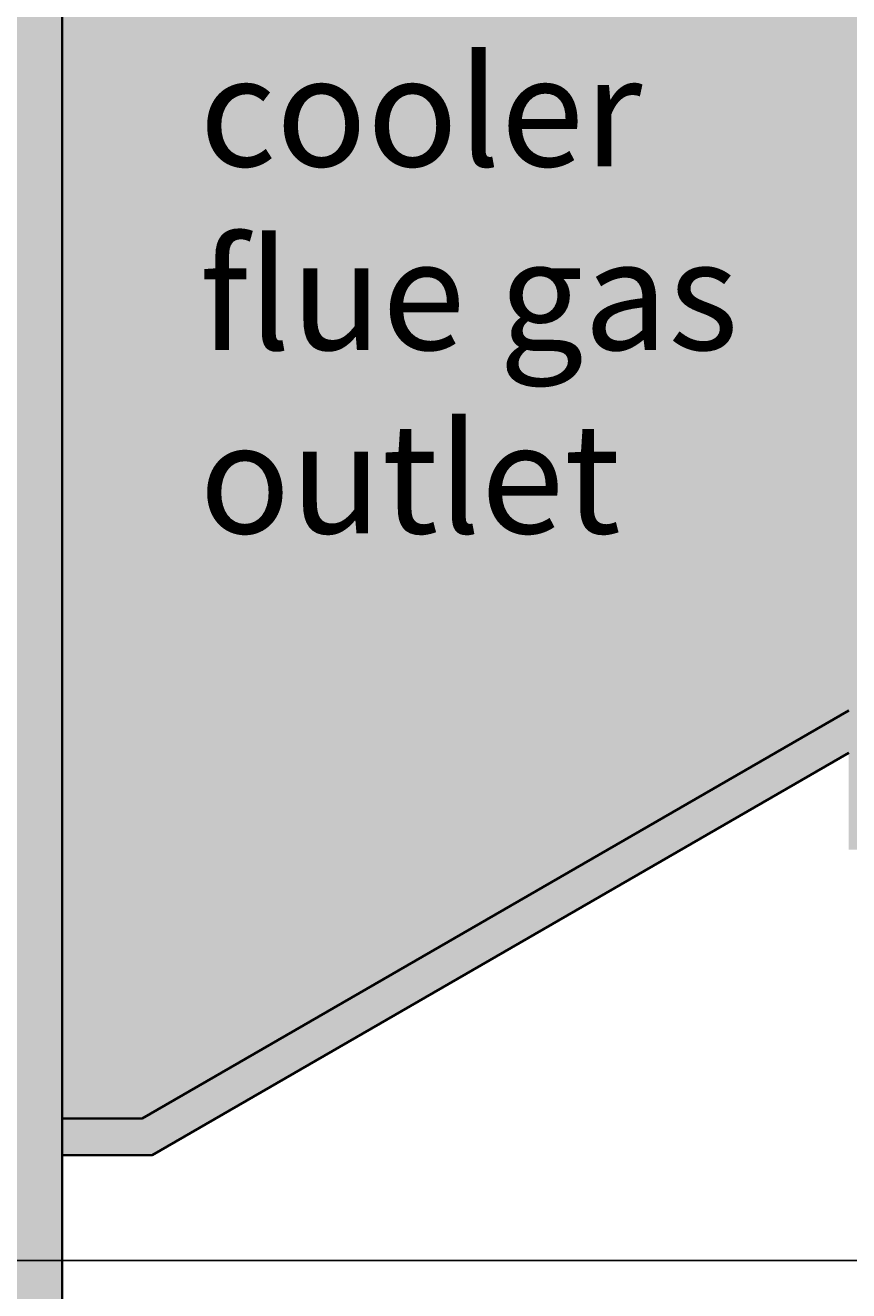
# Model space of a CAD drawing. Units: inches. Extents: x -1 to 292, y -3 to 199.
# Tile 38 of 52: x 181 to 203, y 43 to 77. Entities that reach past the tile are written whole.
import ezdxf

# ---------------------------------------------------------------- set-up
doc = ezdxf.new("R2010")
doc.units = ezdxf.units.IN
doc.header["$MEASUREMENT"] = 0
for name, color, linetype, lineweight in [('M-ANNO-TEXT', 3, 'Continuous', 25), ('M-DIMS', 2, 'Continuous', 18), ('M-EQPM', 7, 'Continuous', 35), ('M-PATT', 8, 'Continuous', 13)]:
    doc.layers.add(name, color=color, linetype=linetype, lineweight=lineweight)
doc.styles.get("Standard").update_dxf_attribs({"font": 'arial.ttf'})
doc.dimstyles.get("Standard").update_dxf_attribs({"dimtxt": 0.18, "dimasz": 0.18, "dimexe": 0.18, "dimexo": 0.0625, "dimgap": 0.09, "dimtad": 0, "dimtih": 1, "dimtoh": 1, "dimdec": 4, "dimzin": 0, "dimdsep": 46, "dimtxsty": 'Standard', "dimcen": 0.09, "dimadec": 0, "dimazin": 0, "dimtfac": 1, "dimtdec": 4, "dimtofl": 0, "dimtmove": 0, "dimatfit": 3, "dimfxl": 1, "dimtolj": 1, "dimtzin": 0, "dimarcsym": 0})

# ---------------------------------------------------------------- blocks, each defined once
blk = doc.blocks.new('*D7')
at = {"layer": 'Defpoints', "color": 0, "transparency": 16777216}
for p in [(21.861, 54.582), (205.115, 54.582), (21.861, 39.982)]:
    blk.add_point(p, dxfattribs=at)
at = {"layer": 'M-DIMS', "color": 0, "lineweight": -2, "transparency": 16777216}
for p, q in [((21.861, 54.52), (21.861, 39.802)), ((205.115, 54.52), (205.115, 39.802)), ((22.041, 39.982), (113.033, 39.982)), ((204.935, 39.982), (113.944, 39.982))]:
    blk.add_line(p, q, dxfattribs=at)
at = {"layer": 'M-DIMS', "color": 0, "transparency": 16777216}
for points in [[(22.041, 40.012), (22.041, 39.952), (21.861, 39.982)], [(204.935, 40.012), (204.935, 39.952), (205.115, 39.982)]]:
    blk.add_solid(points, dxfattribs=at)
at = {"layer": 'M-DIMS', "color": 0, "transparency": 16777216, "insert": (113.488, 39.982), "char_height": 0.18, "attachment_point": 5}
blk.add_mtext('\\A1;183.25', dxfattribs=at)
blk = doc.blocks.new('*D10')
at = {"layer": 'Defpoints', "color": 0, "transparency": 16777216}
for p in [(169.176, 99.774), (169.176, 43.391), (292.04, 43.391)]:
    blk.add_point(p, dxfattribs=at)
at = {"layer": 'M-DIMS', "color": 0, "lineweight": -2, "transparency": 16777216}
for p, q in [((169.239, 99.774), (292.22, 99.774)), ((292.04, 99.594), (292.04, 71.764)), ((292.04, 43.571), (292.04, 71.4)), ((169.239, 43.391), (292.22, 43.391))]:
    blk.add_line(p, q, dxfattribs=at)
at = {"layer": 'M-DIMS', "color": 0, "transparency": 16777216}
for points in [[(292.01, 99.594), (292.07, 99.594), (292.04, 99.774)], [(292.01, 43.571), (292.07, 43.571), (292.04, 43.391)]]:
    blk.add_solid(points, dxfattribs=at)
at = {"layer": 'M-DIMS', "color": 0, "transparency": 16777216, "insert": (292.04, 71.582), "char_height": 0.18, "attachment_point": 5}
blk.add_mtext('\\A1;56.38', dxfattribs=at)

msp = doc.modelspace()

# ---------------------------------------------------------------- hatches: boundary and pattern name
at = {"layer": 'M-PATT'}
h = msp.add_hatch(color=256, dxfattribs=at)
h.set_gradient(color1=(0, 127, 0), color2=(0, 127, 0), tint=1, name='CYLINDER')
h.paths.add_polyline_path([(164.5186, 119.2985), (129.9293, 119.2985), (129.9293, 117.2985), (164.1897, 117.2985)])
h.paths.add_polyline_path([(181.5897, 119.2985), (164.5186, 119.2985), (164.1897, 117.2985), (179.5897, 117.2985), (179.5897, 107.8518), (181.5897, 109.1506)])
h.paths.add_polyline_path([(181.5897, 109.1506), (179.5897, 107.8518), (179.5897, 36.2698), (198.4159, 36.2698), (198.4159, 38.2698), (181.5897, 38.2698)])
h.paths.add_polyline_path([(115.4883, 126.765), (111.4883, 126.765), (111.4883, 114.6589), (115.4883, 114.6589)])
h.paths.add_polyline_path([(123.408, 119.2985), (115.4883, 119.2985), (115.4883, 117.2985), (123.408, 117.2985)])
h.paths.add_polyline_path([(115.4883, 112.6589), (111.4883, 112.6589), (111.4883, 106.9941), (115.4883, 106.9941)])
h.paths.add_polyline_path([(120.9032, 106.9941), (106.0735, 106.9941), (106.0735, 105.9941), (120.9032, 105.9941)])
h.paths.add_polyline_path([(236.4209, 117.5104), (234.9209, 117.5104), (234.9209, 97.1861), (236.4209, 97.1861)])
h.paths.add_polyline_path([(236.4209, 126.4904), (234.9209, 126.4904), (234.9209, 118.9331), (236.4209, 118.9331)])
h.paths.add_polyline_path([(244.9552, 125.7269), (242.9552, 125.7269), (242.9552, 116.8562), (244.9552, 116.8562)])
h.paths.add_polyline_path([(244.9552, 115.1721), (242.9552, 115.1721), (242.9552, 109.7385), (244.9552, 109.7385)])
h.paths.add_polyline_path([(248.4468, 109.7385), (239.4637, 109.7385), (239.4637, 109.4289), (248.4468, 109.4289)])
h = msp.add_hatch(color=256, dxfattribs=at)
h.set_gradient(color1=(237, 31, 36), color2=(242, 113, 114), tint=1, name='CYLINDER')
h.paths.add_polyline_path([(106.0735, 105.9941), (106.0735, 106.9941), (108.0603, 106.9941), (107.8488, 107.6501), (57.8007, 107.6501, 0.4142136), (49.9241, 99.7735), (52.3176, 101.3278), (55.0097, 99.7735), (57.4032, 101.3278), (60.0953, 99.7735), (62.4888, 101.3278), (65.1809, 99.7735), (67.5744, 101.3278), (70.2665, 99.7735), (72.66, 101.3278), (75.3521, 99.7735), (77.7456, 101.3278), (80.4377, 99.7735), (82.8312, 101.3278), (85.5233, 99.7735), (87.9168, 101.3278), (90.6089, 99.7735), (93.0024, 101.3278), (95.6945, 99.7735), (98.088, 101.3278), (100.7801, 99.7735), (103.1736, 101.3278), (105.8657, 99.7735), (108.2592, 101.3278), (110.9513, 99.7735), (113.3448, 101.3278), (116.0369, 99.7735), (118.4304, 101.3278), (121.1225, 99.7735), (123.516, 101.3278), (126.2082, 99.7735), (128.6016, 101.3278), (131.2938, 99.7735), (133.6872, 101.3278), (136.3794, 99.7735), (138.7728, 101.3278), (141.465, 99.7735), (143.8584, 101.3278), (146.5506, 99.7735), (148.944, 101.3278), (151.6362, 99.7735), (154.0296, 101.3278), (156.7218, 99.7735), (159.1152, 101.3278), (160.6222, 100.4578), (160.6222, 107.6501), (115.4883, 107.6501), (115.4883, 106.9941), (120.9032, 106.9941), (120.9032, 105.9941), (120.9032, 103.3981), (106.0735, 103.3981)])
h.paths.add_polyline_path([(169.176, 107.6501), (162.1623, 107.6501), (162.1623, 100.004), (164.2008, 101.3278), (166.893, 99.7735), (169.2864, 101.3278), (171.9786, 99.7735), (174.372, 101.3278), (177.0526, 99.7802, 0.4139642)])
h.paths.add_polyline_path([(111.4883, 107.6501), (107.8488, 107.6501), (108.0603, 106.9941), (111.4883, 106.9941)], flags=17)
h.paths.add_polyline_path([(61.6788, 91.897), (57.8007, 91.897, -0.1099266), (54.4604, 92.6403), (43.2011, 92.6403), (23.9502, 84.4688), (23.9502, 58.376), (43.2011, 47.2615), (50.9409, 47.2615, -0.2705926), (57.8007, 51.2672), (61.6788, 51.2672)])
h.paths.add_polyline_path([(73.6788, 91.897), (70.6788, 91.897), (70.6788, 51.2672), (73.6788, 51.2672)])
h.paths.add_polyline_path([(79.6788, 91.897), (76.6788, 91.897), (76.6788, 51.2672), (79.6788, 51.2672)])
h.paths.add_polyline_path([(67.6788, 91.897), (64.6788, 91.897), (64.6788, 51.2672), (67.6788, 51.2672)])
h.paths.add_polyline_path([(101.6788, 91.897), (82.6788, 91.897), (82.6788, 51.2672), (101.6788, 51.2672)])
h.paths.add_polyline_path([(107.6788, 91.897), (104.6788, 91.897), (104.6788, 51.2672), (107.6788, 51.2672)])
h.paths.add_polyline_path([(113.6788, 91.897), (110.6788, 91.897), (110.6788, 51.2672), (113.6788, 51.2672)])
h.paths.add_polyline_path([(119.6788, 91.897), (116.6788, 91.897), (116.6788, 51.2672), (119.6788, 51.2672)])
h.paths.add_polyline_path([(141.6788, 91.897), (122.6788, 91.897), (122.6788, 51.2672), (141.6788, 51.2672)])
h.paths.add_polyline_path([(147.6788, 91.897), (144.6788, 91.897), (144.6788, 51.2672), (147.6788, 51.2672)])
h.paths.add_polyline_path([(153.6788, 91.897), (150.6788, 91.897), (150.6788, 51.2672), (153.6788, 51.2672)])
h.paths.add_polyline_path([(159.6788, 91.897), (156.6788, 91.897), (156.6788, 51.2672), (159.6788, 51.2672)])
h.paths.add_polyline_path([(179.5897, 92.6403), (172.5163, 92.6403, -0.1099266), (169.176, 91.897), (162.6788, 91.897), (162.6788, 51.2672), (169.176, 51.2672, -0.2705926), (176.0358, 47.2615), (179.5897, 47.2615)])
h.paths.add_polyline_path([(203.0265, 84.4688), (183.7755, 92.6403), (181.5897, 92.6403), (181.5897, 47.2615), (183.7755, 47.2615), (203.0265, 58.376)])
h.paths.add_polyline_path([(184.4188, 61.52), (200.7224, 61.52), (200.7224, 77.7532), (184.4188, 77.7532)], flags=24)
h = msp.add_hatch(color=256, dxfattribs=at)
h.set_gradient(color1=(76, 38, 47), color2=(76, 38, 47), tint=1, name='CYLINDER')
h.paths.add_polyline_path([(40.8628, 91.6478), (40.3591, 92.5203), (23.9502, 85.5552), (23.9502, 84.4688)])
h.paths.add_polyline_path([(52.8586, 93.6403), (42.9977, 93.6403), (40.3591, 92.5203), (40.8628, 91.6478), (43.2011, 92.6403), (54.4604, 92.6403, -0.0601508)])
h.paths.add_polyline_path([(23.9502, 88.5821), (21.8612, 88.5821), (21.8612, 54.5821), (23.9502, 54.5821)])
h.paths.add_polyline_path([(23.9502, 58.376), (23.9502, 57.2213), (42.9332, 46.2615), (50.4659, 46.2615, -0.0351813), (50.9409, 47.2615), (43.2011, 47.2615)])
h.paths.add_polyline_path([(179.5897, 93.6403), (174.1181, 93.6403, -0.0601508), (172.5163, 92.6403), (179.5897, 92.6403)])
h.paths.add_polyline_path([(183.979, 93.6403), (181.5897, 93.6403), (181.5897, 92.6403), (183.7755, 92.6403), (203.0265, 84.4688), (203.0265, 85.5552)])
h.paths.add_polyline_path([(205.1155, 88.5821), (203.0265, 88.5821), (203.0265, 54.5821), (205.1155, 54.5821)])
h.paths.add_polyline_path([(203.0265, 57.2213), (203.0265, 58.376), (183.7755, 47.2615), (181.5897, 47.2615), (181.5897, 46.2615), (184.0435, 46.2615)])
h.paths.add_polyline_path([(179.5897, 47.2615), (176.0358, 47.2615, -0.0351813), (176.5107, 46.2615), (179.5897, 46.2615)])

# ---------------------------------------------------------------- linework, layer by layer
at = {"layer": 'M-EQPM'}
for points in [[(129.9293, 119.2985), (181.5897, 119.2985), (181.5897, 38.2698)], [(203.0265, 58.376), (183.7755, 47.2615), (181.5897, 47.2615)], [(203.0265, 57.2213), (184.0435, 46.2615), (181.5897, 46.2615)]]:
    msp.add_lwpolyline(points, dxfattribs=at)

# ---------------------------------------------------------------- texts
at = {"layer": 'M-ANNO-TEXT', "insert": (185.3325, 76.2092), "char_height": 3, "attachment_point": 1}
msp.add_mtext_dynamic_manual_height_columns('cooler \\Pflue gas \\Poutlet', width=47.899539, gutter_width=1, heights=[0], dxfattribs=at)

# ---------------------------------------------------------------- dimensions: what is measured, and where the dimension line sits
at = {"layer": 'M-DIMS'}
for base, p1, p2, angle, picture, middle in [((292.0399, 43.3906), (169.176, 99.7735), (169.176, 43.3906), 90, '*D10', (292.0399, 71.5821)), ((21.8612, 39.9821), (205.1155, 54.5821), (21.8612, 54.5821), 180, '*D7', (113.4883, 39.9821))]:
    dim = msp.add_linear_dim(base=base, p1=p1, p2=p2, angle=angle, dimstyle='Standard', override={"dimdec": 2, "dimlfac": 1, "dimrnd": 0, "dimzin": 0, "dimdsep": 46, "dimlunit": 2}, dxfattribs=at)
    dim.commit()
    dim.dimension.update_dxf_attribs({"geometry": picture, "text_midpoint": middle})

doc.saveas('drawing.dxf')
